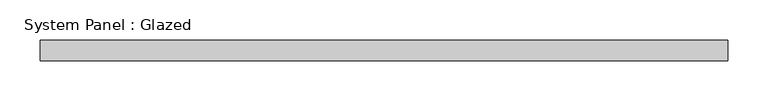
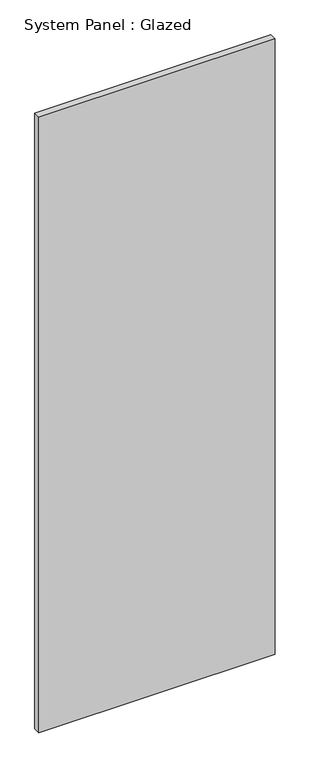
"""IFC4 building model written with IfcOpenShell, lengths in millimetres: plate geometry, System Panel : Glazed."""

from ifc_helpers import new_model, si_unit, origin, origin_with_axes, place, context, project, spatial, polyline, outline, extrude, source, transform, mapped, element, save


def system_panel_glazed_ea0d7bad(model_context):
    return source(origin(), model_context, "Body", "SweptSolid", [
        extrude(outline(polyline([(425.4499999, 19.05), (-425.4499999, 19.05), (-425.4499999, 44.45), (425.4499999, 44.45), (425.4499999, 19.05)])), origin_with_axes(), (0.0, 0.0, 1.0), 2343.15),
    ])


if __name__ == "__main__":
    model = new_model("IFC4")
    model_context = context("Model", 3, world=origin())
    ifc_project = project(units=[si_unit("LENGTHUNIT", "METRE", prefix="MILLI")], contexts=[model_context])
    site = spatial("IfcSite", under=ifc_project)
    building = spatial("IfcBuilding", under=site)
    placement = place(None, origin())
    system_panel_glazed_shape = system_panel_glazed_ea0d7bad(model_context)
    element("IfcPlate", 1, ObjectType="System Panel : Glazed", at=placement, inside=building, context=model_context, shape_type="MappedRepresentation", body=[
        mapped(system_panel_glazed_shape, transform((0.0, 0.0, 0.0), x_axis=(1.0, 0.0, 0.0), y_axis=(0.0, 1.0, 0.0), z_axis=(0.0, 0.0, 1.0))),
    ])
    save(model, "model.ifc")

# Revit data of these elements
# Type "System Panel : Glazed"
#   Construction Type Id = "GSP4R"
#   Analytic Construction = "1/8 in Pilkington single glazing"
#   Visual Light Transmittance = 0.9
#   Solar Heat Gain Coefficient = 0.86
#   Heat Transfer Coefficient (U) = 1.18115 BTU/(h·ft²·°F)
#   Define Thermal Properties by = 1
# Element 1 (IfcPlate, "System Panel : Glazed")
#   Materials on its faces: "Glass"
# Materials
#   "Glass": class "Glass", colour RGB 0 128 192, transparency 0.75, Description = "Soda Lime Glass", Cost = 0
